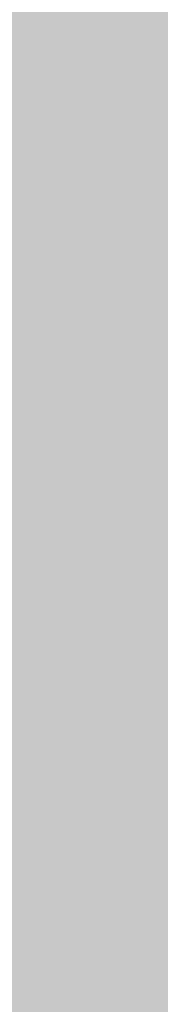
# Model space of a CAD drawing. Units: inches. Extents: x 2083 to 3317, y 1141 to 2115.
# Tile 188 of 256: x 3126.8914 to 3126.9283, y 1263.3548 to 1263.6134. Entities that reach past the tile are written whole.
import ezdxf

# ---------------------------------------------------------------- set-up
doc = ezdxf.new("R2010")
doc.units = ezdxf.units.IN
doc.layers.add('A-ANNO-DIMS', color=2, linetype='Continuous', lineweight=18)
doc.layers.add('A-WALL-PATT', color=251, linetype='Continuous', lineweight=13, true_color=0x636466)
doc.styles.get("Standard").update_dxf_attribs({"font": 'arial.ttf'})
doc.dimstyles.new('ISO-25', dxfattribs={"dimtxt": 12, "dimasz": 12, "dimexe": 1.25, "dimexo": 0.625, "dimtad": 1, "dimlunit": 3, "dimtxsty": 'Standard', "dimcen": 2.5, "dimadec": 0, "dimazin": 0, "dimtfac": 1, "dimtmove": 0, "dimatfit": 3, "dimfxl": 1, "dimarcsym": 0})

# ---------------------------------------------------------------- blocks, each defined once
blk = doc.blocks.new('*D26')
at = {"layer": 'A-ANNO-DIMS', "color": 0, "lineweight": -2, "transparency": 16777216}
for p, q in [((3088.98584, 1274.91509), (3088.98584, 1270.95196)), ((3111.24004, 1274.91509), (3111.24004, 1270.95196)), ((3076.98584, 1272.20196), (2840.26245, 1272.20196)), ((3111.24004, 1272.20196), (3088.98584, 1272.20196)), ((3123.24004, 1272.20196), (3135.24004, 1272.20196))]:
    blk.add_line(p, q, dxfattribs=at)
at = {"layer": 'A-ANNO-DIMS', "color": 0, "transparency": 16777216}
for points in [[(3076.98584, 1274.20196), (3076.98584, 1270.20196), (3088.98584, 1272.20196)], [(3123.24004, 1274.20196), (3123.24004, 1270.20196), (3111.24004, 1272.20196)]]:
    blk.add_solid(points, dxfattribs=at)
at = {"layer": 'Defpoints', "color": 0, "transparency": 16777216}
for p in [(3088.98584, 1275.54009), (3111.24004, 1275.54009), (3088.98584, 1272.20196)]:
    blk.add_point(p, dxfattribs=at)
at = {"layer": 'A-ANNO-DIMS', "color": 0, "transparency": 16777216, "insert": (2952.62415, 1279.0316), "char_height": 12, "attachment_point": 5}
blk.add_mtext('NIGHTSTAND 1\'-10 1/2" TYP.', dxfattribs=at)
blk = doc.blocks.new('*D27')
at = {"layer": 'A-ANNO-DIMS', "color": 0, "lineweight": -2, "transparency": 16777216}
for p, q in [((3114.57817, 1309.79428), (3114.57817, 1321.79428)), ((3111.86504, 1297.79428), (3115.82817, 1297.79428)), ((3114.57817, 1297.79428), (3114.57817, 1275.54009)), ((3111.86504, 1275.54009), (3115.82817, 1275.54009)), ((3114.57817, 1263.54009), (3114.57817, 1140.98859))]:
    blk.add_line(p, q, dxfattribs=at)
at = {"layer": 'A-ANNO-DIMS', "color": 0, "transparency": 16777216}
for points in [[(3112.57817, 1309.79428), (3116.57817, 1309.79428), (3114.57817, 1297.79428)], [(3112.57817, 1263.54009), (3116.57817, 1263.54009), (3114.57817, 1275.54009)]]:
    blk.add_solid(points, dxfattribs=at)
at = {"layer": 'Defpoints', "color": 0, "transparency": 16777216}
for p in [(3111.24004, 1297.79428), (3111.24004, 1275.54009), (3114.57817, 1275.54009)]:
    blk.add_point(p, dxfattribs=at)
at = {"layer": 'A-ANNO-DIMS', "color": 0, "transparency": 16777216, "insert": (3107.74853, 1196.26434), "char_height": 12, "attachment_point": 5, "rotation": 90}
blk.add_mtext('1\'-10 1/2" TYP.', dxfattribs=at)

msp = doc.modelspace()

# ---------------------------------------------------------------- hatches: boundary and pattern name
at = {"layer": 'A-WALL-PATT'}
h = msp.add_hatch(color=256, dxfattribs=at)
h.dxf.hatch_style = 1
h.paths.add_polyline_path([(3126.95978, 2020.76136), (2748.95978, 2020.76136), (2604.95978, 2020.76136), (2226.95978, 2020.76136), (2226.95978, 1702.76136), (2466.95978, 1702.76136), (2466.95978, 1582.76136), (2418.95978, 1582.76136), (2418.95978, 1477.76136), (2226.95978, 1477.76136), (2226.95978, 1263.26136), (2544.95978, 1263.26136), (2544.95978, 1411.76136), (2604.95978, 1411.76136), (2685.95978, 1411.76136), (2685.95978, 1420.76136), (2604.95978, 1420.76136), (2604.95978, 1573.76136), (2604.95978, 1702.76136), (2604.95978, 2011.76136), (2748.95978, 2011.76136), (2748.95978, 1702.76136), (2862.95978, 1702.76136), (2862.95978, 1621.76136), (2871.95978, 1621.76136), (2871.95978, 1702.76136), (2883.95978, 1702.76136), (2883.95978, 1706.93946, -0.026459), (2883.95978, 1711.76136), (2757.95978, 1711.76136), (2757.95978, 1807.76136), (2787.95978, 1807.76136), (2787.95978, 1812.26136), (2757.95978, 1812.26136), (2757.95978, 2011.76136), (2877.95978, 2011.76136), (2877.95978, 1812.26136), (2847.95978, 1812.26136), (2847.95978, 1807.76136), (2889.83574, 1807.76136), (2889.83574, 1812.26136), (2882.45978, 1812.26136), (2882.45978, 2011.76136), (3117.95978, 2011.76136), (3117.95978, 1812.26136), (2937.83574, 1812.26136), (2937.83574, 1807.76136), (2995.70978, 1807.76136), (2995.70978, 1796.11767), (3000.20978, 1796.11767), (3000.20978, 1807.76136), (3117.95978, 1807.76136), (3117.95978, 1711.76136), (3000.20978, 1711.76136), (3000.20978, 1760.11767), (2998.5727, 1760.11767, -0.020711), (2995.70978, 1760.11767), (2995.70978, 1711.76136), (2931.95978, 1711.76136), (2931.95978, 1702.76136), (3126.95978, 1702.76136)])
h.paths.add_polyline_path([(2471.45978, 2011.76136), (2471.45978, 1810.01136), (2462.71694, 1810.01136), (2462.71694, 1805.51136), (2505.95978, 1805.51136), (2505.95978, 1810.01136), (2475.95978, 1810.01136), (2475.95978, 2011.76136), (2595.95978, 2011.76136), (2595.95978, 1810.01136), (2565.95978, 1810.01136), (2565.95978, 1805.51136), (2595.95978, 1805.51136), (2595.95978, 1711.76136), (2235.95978, 1711.76136), (2235.95978, 1805.51136), (2353.70978, 1805.51136), (2353.70978, 1796.05416), (2358.20978, 1796.05416), (2358.20978, 1805.51136), (2414.71694, 1805.51136), (2414.71694, 1810.01136), (2235.95978, 1810.01136), (2235.95978, 2011.76136)], flags=16)
h.paths.add_polyline_path([(2270.20473, 1994.61001), (2270.20473, 1970.61001), (2246.20473, 1970.61001), (2246.20473, 1994.61001)], flags=0)
edge = h.paths.add_edge_path(flags=0)
edge.add_ellipse((2332.02739, 1899.79818), major_axis=(-3.04299, 3.04299), ratio=0.1682525, start_angle=-161.33217, end_angle=-156.30711, ccw=False)
edge.add_ellipse((2333.08204, 1898.74353), major_axis=(-1.05465, 1.05465), ratio=0.4535321, start_angle=-123.37102, end_angle=-94.15911)
edge = h.paths.add_edge_path(flags=0)
edge.add_ellipse((2332.02739, 1968.87629), major_axis=(3.04299, 3.04299), ratio=0.1682525, start_angle=18.66783, end_angle=23.69289)
edge.add_spline(control_points=[(2332.9256, 1970.6911), (2332.22677, 1970.3361), (2330.89371, 1969.65891), (2328.41308, 1970.93214), (2327.20393, 1967.74871), (2324.7096, 1969.95559), (2322.53282, 1967.01235), (2320.01285, 1971.29581), (2317.68031, 1968.15784), (2316.04053, 1967.10205), (2315.4269, 1966.8096)], knot_values=[0, 0, 0, 0, 2.267059, 4.324559, 6.685584, 8.878641, 11.121502, 14.300359, 17.755284, 19.732645, 19.732645, 19.732645, 19.732645], degree=3, periodic=0)
edge.add_ellipse((2332.02739, 1968.87629), major_axis=(3.04299, 3.04299), ratio=0.1682525, start_angle=18.66783, end_angle=23.69289, ccw=False)
edge.add_ellipse((2333.08204, 1969.93094), major_axis=(1.05465, 1.05465), ratio=0.4535321, start_angle=56.62898, end_angle=85.84089, ccw=False)
edge = h.paths.add_edge_path(flags=0)
edge.add_spline(control_points=[(2296.42829, 1967.98791), (2293.6278, 1965.33631), (2287.70362, 1959.72709), (2299.74386, 1949.9957), (2294.53259, 1935.66853), (2290.57323, 1920.60351), (2293.39412, 1909.97369), (2296.18541, 1904.96654)], knot_values=[0.099185, 0.099185, 0.099185, 0.099185, 0.345301, 0.619822, 0.982653, 1.386093, 1.810555, 1.810555, 1.810555, 1.810555], degree=3, periodic=0)
edge.add_spline(control_points=[(2296.18541, 1904.96654), (2297.38358, 1902.6193), (2298.00097, 1901.94931), (2298.55297, 1901.46815)], knot_values=[0.006246, 0.006246, 0.006246, 0.006246, 0.055476, 0.055476, 0.055476, 0.055476], degree=3, periodic=0)
edge.add_spline(control_points=[(2298.55297, 1901.46815), (2297.25861, 1900.92322), (2295.22529, 1900.23213), (2293.06023, 1900.61421), (2292.10142, 1900.78841), (2292.08958, 1900.79057)], knot_values=[0.312835, 0.312835, 0.312835, 0.312835, 0.40178, 0.474987, 0.475903, 0.475903, 0.475903, 0.475903], degree=3, periodic=0)
edge.add_arc((2292.79365, 1904.66411), 3.93701, 215.4209, 259.69818, ccw=False)
edge.add_spline(control_points=[(2289.58531, 1902.3823), (2289.47665, 1902.53509), (2289.36848, 1902.68804), (2289.26086, 1902.84117)], knot_values=[0.102872, 0.102872, 0.102872, 0.102872, 0.116896, 0.116896, 0.116896, 0.116896], degree=3, periodic=0)
edge.add_spline(control_points=[(2289.26086, 1902.84117), (2288.6866, 1902.55019), (2287.64005, 1902.0199), (2285.88134, 1901.87395), (2283.85297, 1901.50435), (2281.71999, 1899.71054), (2278.46699, 1899.49294), (2276.15714, 1901.8832), (2272.25895, 1899.80407), (2267.77761, 1901.84318), (2262.24388, 1900.18403), (2257.41493, 1901.78206), (2254.31837, 1900.72612), (2253.17828, 1900.33734)], knot_values=[0, 0, 0, 0, 1.907977, 3.477176, 5.261074, 7.972851, 11.680248, 13.717921, 16.939592, 22.789562, 27.502503, 33.595215, 37.145618, 37.145618, 37.145618, 37.145618], degree=3, periodic=0)
edge.add_line((2253.17828, 1900.33734), (2250.24424, 1902.84117))
edge.add_line((2250.24424, 1902.84117), (2250.24424, 1965.8333))
edge.add_line((2250.24424, 1965.8333), (2253.17828, 1968.33712))
edge.add_spline(control_points=[(2253.17828, 1968.33712), (2254.31837, 1967.94835), (2257.41493, 1966.89241), (2262.24388, 1968.49043), (2267.77761, 1966.83128), (2271.52673, 1968.53722), (2273.87591, 1967.82829), (2274.2067, 1967.72764)], knot_values=[0, 0, 0, 0, 0.09018, 0.244935, 0.364644, 0.513233, 0.537855, 0.537855, 0.537855, 0.537855], degree=3, periodic=0)
edge.add_arc((2274.35289, 1963.79335), 3.93701, 72.05113, 92.12795, ccw=False)
edge.add_arc((2281.29693, 1985.23), 18.5963, 252.051134, 288.565722)
edge.add_arc((2292.31672, 1956.02888), 12.64608, 71.026788, 113.778218, ccw=False)
edge = h.paths.add_edge_path(flags=0)
edge.add_spline(control_points=[(2274.89941, 1951.85619), (2275.06616, 1951.61659), (2275.23269, 1951.37659), (2275.39799, 1951.13585)], knot_values=[1.409916, 1.409916, 1.409916, 1.409916, 1.43159, 1.43159, 1.43159, 1.43159], degree=3, periodic=0)
edge.add_spline(control_points=[(2275.39799, 1951.13585), (2275.79211, 1950.56189), (2276.17923, 1949.98377), (2276.54555, 1949.3971)], knot_values=[1.358238, 1.358238, 1.358238, 1.358238, 1.409916, 1.409916, 1.409916, 1.409916], degree=3, periodic=0)
edge.add_line((2276.54555, 1949.3971), (2277.43729, 1947.86218))
edge.add_spline(control_points=[(2277.43729, 1947.86218), (2276.30383, 1945.67311), (2274.6397, 1942.42688), (2274.63161, 1938.0939), (2272.79912, 1930.85155), (2274.35643, 1943.89705), (2275.94768, 1947.92336), (2276.54555, 1949.3971)], knot_values=[0.005632, 0.005632, 0.005632, 0.005632, 0.186014, 0.266002, 0.357087, 0.59639, 0.739732, 0.739732, 0.739732, 0.739732], degree=3, periodic=0)
edge.add_spline(control_points=[(2276.54555, 1949.3971), (2276.17923, 1949.98377), (2275.79211, 1950.56189), (2275.39799, 1951.13585)], knot_values=[1.358238, 1.358238, 1.358238, 1.358238, 1.409916, 1.409916, 1.409916, 1.409916], degree=3, periodic=0)
edge.add_spline(control_points=[(2275.39799, 1951.13585), (2274.9425, 1950.08045), (2274.20776, 1948.02527), (2273.9346, 1944.85148), (2272.46853, 1937.62749), (2273.46622, 1945.69647), (2274.70062, 1951.05947), (2274.89941, 1951.85619)], knot_values=[0.104364, 0.104364, 0.104364, 0.104364, 0.189636, 0.269624, 0.36071, 0.600013, 0.644622, 0.644622, 0.644622, 0.644622], degree=3, periodic=0)
h.paths.add_polyline_path([(2269.16751, 1963.12757, -0.357527), (2268.17063, 1960.97637, -0.092561), (2268.17063, 1939.43632, -0.357527), (2269.16751, 1937.28512, -0.357527), (2267.01631, 1938.282, -0.164785), (2254.68558, 1938.282, -0.357527), (2252.53438, 1937.28512, -0.357527), (2253.53126, 1939.43632, -0.092561), (2253.53126, 1960.97637, -0.357527), (2252.53438, 1963.12757, -0.357527), (2254.68558, 1962.13069, -0.164785), (2267.01631, 1962.13069, -0.357527)], flags=0)
h.paths.add_polyline_path([(2248.87407, 1967.8018), (2248.87407, 1957.02771), (2249.45778, 1957.02771), (2249.45778, 1911.64676), (2248.87407, 1911.64676), (2248.87407, 1900.87267), (2246.51186, 1900.87267, 0.197327), (2244.14966, 1902.45687), (2244.14966, 1966.21759, 0.197327), (2246.51186, 1967.8018)], flags=0)
h.paths.add_polyline_path([(2269.16751, 1931.38934, -0.357527), (2268.17063, 1929.23814, -0.092561), (2268.17063, 1907.6981, -0.357527), (2269.16751, 1905.54689, -0.357527), (2267.01631, 1906.54377, -0.164785), (2254.68558, 1906.54377, -0.357527), (2252.53438, 1905.54689, -0.357527), (2253.53126, 1907.6981, -0.092561), (2253.53126, 1929.23814, -0.357527), (2252.53438, 1931.38934, -0.357527), (2254.68558, 1930.39246, -0.164785), (2267.01631, 1930.39246, -0.357527)], flags=0)
edge = h.paths.add_edge_path(flags=0)
edge.add_spline(control_points=[(2276.19686, 1906.7237), (2276.16814, 1909.02893), (2276.11405, 1913.37185), (2270.59842, 1924.92498), (2273.90517, 1919.01278), (2275.92171, 1916.26206), (2275.47457, 1912.40215), (2277.25787, 1910.38062), (2276.69604, 1908.22504), (2276.64622, 1906.81302), (2276.61782, 1906.00841)], knot_values=[0, 0, 0, 0, 8.61026, 16.221274, 18.843057, 23.804898, 27.440828, 29.356102, 31.203478, 33.650687, 33.650687, 33.650687, 33.650687], degree=3, periodic=0)
edge.add_spline(control_points=[(2276.61782, 1906.00841), (2276.62331, 1905.62414), (2276.49774, 1904.62866), (2275.44178, 1903.85473), (2274.93731, 1903.08045), (2274.85908, 1902.84117)], knot_values=[0.156488, 0.156488, 0.156488, 0.156488, 0.184398, 0.231376, 0.250598, 0.250598, 0.250598, 0.250598], degree=3, periodic=0)
edge.add_line((2274.85908, 1902.84117), (2276.50598, 1902.84117))
edge.add_spline(control_points=[(2276.50598, 1902.84117), (2276.78831, 1903.08494), (2277.66507, 1904.1252), (2278.24954, 1904.34074), (2277.65387, 1908.52739), (2278.15567, 1906.22781), (2278.10046, 1905.28595), (2278.84667, 1904.06901), (2277.85679, 1903.41495), (2277.87419, 1902.99105), (2277.90356, 1902.84117)], knot_values=[0.059574, 0.059574, 0.059574, 0.059574, 0.080753, 0.103741, 0.16972, 0.176036, 0.207137, 0.240474, 0.262341, 0.27366, 0.27366, 0.27366, 0.27366], degree=3, periodic=0)
edge.add_line((2277.90356, 1902.84117), (2280.02983, 1902.84117))
edge.add_spline(control_points=[(2280.02983, 1902.84117), (2279.88822, 1903.0884), (2279.49926, 1903.98155), (2280.15228, 1905.93935), (2278.10362, 1909.65776), (2279.76239, 1907.18529), (2280.3279, 1904.87486), (2280.48511, 1903.48959), (2281.46327, 1903.24943), (2281.75834, 1902.9365), (2281.83404, 1902.84117)], knot_values=[0.013856, 0.013856, 0.013856, 0.013856, 0.034874, 0.088867, 0.107879, 0.126738, 0.158714, 0.193757, 0.217487, 0.226722, 0.226722, 0.226722, 0.226722], degree=3, periodic=0)
edge.add_spline(control_points=[(2281.83404, 1902.84117), (2281.78753, 1902.8267), (2281.64702, 1902.78299), (2281.39553, 1902.85949), (2281.08808, 1902.98524), (2280.72068, 1903.0609), (2280.33345, 1903.02573), (2280.12477, 1902.89888), (2280.02983, 1902.84117)], knot_values=[0, 0, 0, 0, 0.14413, 0.435517, 0.749276, 1.153046, 1.548371, 1.878348, 1.878348, 1.878348, 1.878348], degree=3, periodic=0)
edge.add_line((2280.02983, 1902.84117), (2277.90356, 1902.84117))
edge.add_spline(control_points=[(2277.90356, 1902.84117), (2277.89286, 1902.79586), (2277.8654, 1902.67964), (2277.60748, 1902.68748), (2277.27405, 1902.8007), (2276.83792, 1902.61977), (2276.58381, 1902.78926), (2276.50598, 1902.84117)], knot_values=[0, 0, 0, 0, 0.127189, 0.326199, 0.628009, 1.24357, 1.515331, 1.515331, 1.515331, 1.515331], degree=3, periodic=0)
edge.add_line((2276.50598, 1902.84117), (2274.85908, 1902.84117))
edge.add_spline(control_points=[(2274.85908, 1902.84117), (2274.81444, 1902.89859), (2274.72513, 1903.01345), (2274.49348, 1903.11897), (2274.24429, 1902.96054), (2273.93712, 1903.18494), (2273.61404, 1902.98314), (2273.40832, 1902.88304), (2273.32225, 1902.84117)], knot_values=[0, 0, 0, 0, 0.21843, 0.436957, 0.687977, 0.990379, 1.398396, 1.69185, 1.69185, 1.69185, 1.69185], degree=3, periodic=0)
edge.add_spline(control_points=[(2273.32225, 1902.84117), (2273.61674, 1903.44569), (2274.274, 1904.53825), (2276.02724, 1904.5737), (2276.20696, 1906.58364), (2276.19686, 1906.7237)], knot_values=[0.012227, 0.012227, 0.012227, 0.012227, 0.059472, 0.106218, 0.134458, 0.134458, 0.134458, 0.134458], degree=3, periodic=0)
h.paths.add_polyline_path([(2270.77605, 1897.78983), (2270.77605, 1873.78983), (2246.77605, 1873.78983), (2246.77605, 1897.78983)], flags=0)
h.paths.add_polyline_path([(2353.70978, 1760.00506), (2353.70978, 1760.05416), (2358.20978, 1760.05416, -0.033729)], flags=0)
h.paths.add_polyline_path([(2321.81912, 1737.52919), (2341.99533, 1737.52919, -0.414214), (2343.20327, 1736.32124), (2343.20327, 1721.0206, -0.414214), (2341.99533, 1719.81265), (2321.81912, 1719.81265, -0.414214), (2320.61117, 1721.0206), (2320.61117, 1736.32124, -0.414214)], flags=0)
h.paths.add_polyline_path([(2324.23501, 1736.32124), (2339.57944, 1736.32124, -0.414214), (2341.99533, 1733.90535), (2341.99533, 1725.44973, -0.414214), (2339.57944, 1723.03384), (2333.68059, 1723.03384), (2333.84532, 1722.04547, -0.870646), (2335.4254, 1721.82589, -0.767327), (2333.92269, 1721.42324), (2331.29102, 1721.42324, -0.767327), (2329.78832, 1721.82589, -0.870646), (2331.3684, 1722.04547), (2331.53313, 1723.03384), (2324.23501, 1723.03384, -0.414214), (2321.81912, 1725.44973), (2321.81912, 1733.90535, -0.414214)], flags=0)
h.paths.add_polyline_path([(2570.48379, 1928.61544), (2589.68379, 1928.61544), (2590.16883, 1928.61544), (2590.16883, 1904.9934), (2570.48379, 1904.9934)], flags=0)
h.paths.add_polyline_path([(2574.44732, 1927.26382, -1), (2572.82884, 1927.26382, -1)], flags=0)
h.paths.add_polyline_path([(2573.08987, 1926.94088), (2573.92503, 1927.77604), (2574.14774, 1927.55333), (2573.31258, 1926.71817)], flags=0)
h.paths.add_polyline_path([(2578.77906, 1919.72962, -1), (2571.59166, 1919.72962, -1)], flags=0)
h.paths.add_polyline_path([(2578.38536, 1919.72962, -1), (2571.98536, 1919.72962, -1)], flags=0)
h.paths.add_polyline_path([(2331.59576, 1729.47622, -1), (2333.61795, 1729.47622, -1)], flags=0)
h.paths.add_polyline_path([(2578.03423, 1927.26382, -1), (2576.41574, 1927.26382, -1)], flags=0)
h.paths.add_polyline_path([(2576.68885, 1927.53109), (2576.91156, 1927.7538), (2577.74673, 1926.91863), (2577.52402, 1926.69592)], flags=0)
h.paths.add_polyline_path([(2578.13906, 1909.85954, -1), (2572.23166, 1909.85954, -1)], flags=0)
h.paths.add_polyline_path([(2577.74536, 1909.85954, -1), (2572.62536, 1909.85954, -1)], flags=0)
h.paths.add_polyline_path([(2583.79772, 1927.26382, -1), (2582.17923, 1927.26382, -1)], flags=0)
h.paths.add_polyline_path([(2582.71865, 1927.7538), (2583.55381, 1926.91863), (2583.3311, 1926.69592), (2582.49594, 1927.53109)], flags=0)
h.paths.add_polyline_path([(2582.49594, 1927.53109), (2582.71865, 1927.7538), (2583.55381, 1926.91863), (2583.3311, 1926.69592)], flags=0)
h.paths.add_polyline_path([(2587.73906, 1920.52962, -1), (2581.83166, 1920.52962, -1)], flags=0)
h.paths.add_polyline_path([(2587.34536, 1920.52962, -1), (2582.22536, 1920.52962, -1)], flags=0)
h.paths.add_polyline_path([(2587.38462, 1927.26382, -1), (2585.76613, 1927.26382, -1)], flags=0)
h.paths.add_polyline_path([(2586.08199, 1926.98025), (2586.91716, 1927.81541), (2587.13987, 1927.5927), (2586.3047, 1926.75754)], flags=0)
h.paths.add_polyline_path([(2588.37906, 1910.65954, -1), (2581.19166, 1910.65954, -1)], flags=0)
h.paths.add_polyline_path([(2587.98536, 1910.65954, -1), (2581.58536, 1910.65954, -1)], flags=0)
h.paths.add_polyline_path([(2417.16773, 1729.4779), (2437.34394, 1729.4779, -0.414214), (2438.55188, 1728.26995), (2438.55188, 1712.96931, -0.414214), (2437.34394, 1711.76136), (2417.16773, 1711.76136, -0.414214), (2415.95978, 1712.96931), (2415.95978, 1728.26995, -0.414214)], flags=0)
h.paths.add_polyline_path([(2419.58362, 1728.26995), (2434.92805, 1728.26995, -0.414214), (2437.34394, 1725.85406), (2437.34394, 1717.39844, -0.414214), (2434.92805, 1714.98255), (2429.0292, 1714.98255), (2429.19393, 1713.99418, -0.870646), (2430.77401, 1713.7746, -0.767327), (2429.2713, 1713.37195), (2426.63963, 1713.37195, -0.767327), (2425.13693, 1713.7746, -0.870646), (2426.71701, 1713.99418), (2426.88174, 1714.98255), (2419.58362, 1714.98255, -0.414214), (2417.16773, 1717.39844), (2417.16773, 1725.85406, -0.414214)], flags=0)
h.paths.add_polyline_path([(2419.58362, 1728.26995), (2434.92805, 1728.26995, -0.414214), (2437.34394, 1725.85406), (2437.34394, 1717.39844, -0.414214), (2434.92805, 1714.98255), (2429.0292, 1714.98255), (2428.35812, 1719.00903), (2427.55282, 1719.00903), (2426.88174, 1714.98255), (2419.58362, 1714.98255, -0.414214), (2417.16773, 1717.39844), (2417.16773, 1725.85406, -0.414214)], flags=0)
h.paths.add_polyline_path([(2426.94437, 1721.42492, -1), (2428.96656, 1721.42492, -1)], flags=0)
h.paths.add_polyline_path([(2475.95978, 1702.76136), (2595.95978, 1702.76136), (2595.95978, 1582.76136), (2475.95978, 1582.76136)], flags=16)
h.paths.add_polyline_path([(2427.95978, 1573.76136), (2595.95978, 1573.76136), (2595.95978, 1468.76136), (2595.95978, 1420.76136), (2384.45978, 1420.76136), (2384.45978, 1468.76136), (2427.95978, 1468.76136)], flags=16)
h.paths.add_polyline_path([(2379.95978, 1468.76136), (2379.95978, 1420.76136), (2235.95978, 1420.76136), (2235.95978, 1468.76136)], flags=16)
h.paths.add_polyline_path([(2317.816, 1466.69577), (2337.9922, 1466.69577, -0.414214), (2339.20015, 1465.48782), (2339.20015, 1450.18718, -0.414214), (2337.9922, 1448.97923), (2317.816, 1448.97923, -0.414214), (2316.60805, 1450.18718), (2316.60805, 1465.48782, -0.414214)], flags=0)
h.paths.add_polyline_path([(2320.23189, 1465.48782), (2335.57631, 1465.48782, -0.414214), (2337.9922, 1463.07193), (2337.9922, 1454.61631, -0.414214), (2335.57631, 1452.20042), (2329.67747, 1452.20042), (2329.84219, 1451.21205, -0.870646), (2331.42228, 1450.99247, -0.767327), (2329.91957, 1450.58983), (2327.2879, 1450.58983, -0.767327), (2325.7852, 1450.99247, -0.870646), (2327.36528, 1451.21205), (2327.53001, 1452.20042), (2320.23189, 1452.20042, -0.414214), (2317.816, 1454.61631), (2317.816, 1463.07193, -0.414214)], flags=0)
h.paths.add_polyline_path([(2320.23189, 1465.48782), (2335.57631, 1465.48782, -0.414214), (2337.9922, 1463.07193), (2337.9922, 1454.61631, -0.414214), (2335.57631, 1452.20042), (2329.67747, 1452.20042), (2329.00638, 1456.22691), (2328.20109, 1456.22691), (2327.53001, 1452.20042), (2320.23189, 1452.20042, -0.414214), (2317.816, 1454.61631), (2317.816, 1463.07193, -0.414214)], flags=0)
h.paths.add_polyline_path([(2327.59264, 1458.6428, -1), (2329.61483, 1458.6428, -1)], flags=0)
h.paths.add_polyline_path([(2244.41174, 1433.34045), (2241.92094, 1433.34045, -0.414214), (2240.01786, 1435.24354), (2240.01786, 1440.95281, -0.414211), (2241.92093, 1442.8559), (2244.41174, 1442.8559, -1.976472)], flags=0)
h.paths.add_polyline_path([(2245.35689, 1434.39754, -0.414214), (2245.35689, 1441.79881, -2.144098)], flags=0)
h.paths.add_polyline_path([(2535.95978, 1416.26136), (2535.95978, 1272.26136), (2235.95978, 1272.26136), (2235.95978, 1416.26136)], flags=16)
h.paths.add_polyline_path([(2260.11956, 1384.29284), (2260.11956, 1362.03865), (2237.86537, 1362.03865), (2237.86537, 1384.29284)], flags=0)
edge = h.paths.add_edge_path(flags=0)
edge.add_line((2318.25185, 1362.0933), (2318.1458, 1362.00097))
edge.add_ellipse((2317.44512, 1360.43104), major_axis=(2.82164, 2.82164), ratio=0.1682525, start_angle=18.66783, end_angle=20.94813, ccw=False)
edge.add_ellipse((2318.42305, 1361.40897), major_axis=(0.97793, 0.97793), ratio=0.4535321, start_angle=56.62898, end_angle=70.2262, ccw=False)
edge = h.paths.add_edge_path(flags=0)
edge.add_line((2319.10737, 1295.57108), (2319.01504, 1295.67713))
edge.add_ellipse((2317.44512, 1296.37781), major_axis=(-2.82164, 2.82164), ratio=0.1682525, start_angle=-161.33217, end_angle=-159.05187, ccw=False)
edge.add_ellipse((2318.42305, 1295.39988), major_axis=(-0.97793, 0.97793), ratio=0.4535321, start_angle=-123.37102, end_angle=-109.7738)
edge = h.paths.add_edge_path(flags=0)
edge.add_spline(control_points=[(2284.21035, 1301.17022), (2284.58069, 1300.44472), (2284.89119, 1299.89202), (2285.15955, 1299.46102)], knot_values=[0.039066, 0.039066, 0.039066, 0.039066, 0.055476, 0.055476, 0.055476, 0.055476], degree=3, periodic=0)
edge.add_line((2285.15955, 1299.46102), (2284.21035, 1301.17022))
edge = h.paths.add_edge_path(flags=0)
edge.add_line((2280.41246, 1297.29801), (2283.36999, 1297.03612))
edge.add_line((2283.36999, 1297.03612), (2286.40569, 1297.92631))
edge.add_spline(control_points=[(2286.40569, 1297.92631), (2285.30549, 1297.46312), (2284.34478, 1297.12915), (2283.36999, 1297.03612)], knot_values=[0.394369, 0.394369, 0.394369, 0.394369, 0.475903, 0.475903, 0.475903, 0.475903], degree=3, periodic=0)
edge.add_spline(control_points=[(2283.36999, 1297.03612), (2283.28139, 1297.02767), (2282.31629, 1296.95734), (2281.3125, 1297.13448), (2280.42344, 1297.29602), (2280.41246, 1297.29801)], knot_values=[0.312835, 0.312835, 0.312835, 0.312835, 0.320246, 0.393453, 0.394369, 0.394369, 0.394369, 0.394369], degree=3, periodic=0)
edge = h.paths.add_edge_path(flags=0)
edge.add_line((2284.43556, 1359.60729), (2280.44629, 1355.32805))
edge.add_line((2280.44629, 1355.32805), (2279.57999, 1351.01775))
edge.add_line((2279.57999, 1351.01775), (2282.41297, 1346.58043))
edge.add_spline(control_points=[(2282.41297, 1346.58043), (2283.15333, 1345.58924), (2284.2529, 1344.0289), (2284.80104, 1342.38717), (2284.93516, 1341.80554)], knot_values=[1.240098, 1.240098, 1.240098, 1.240098, 1.332892, 1.382712, 1.382712, 1.382712, 1.382712], degree=3, periodic=0)
edge.add_spline(control_points=[(2284.93516, 1341.80554), (2285.31911, 1340.1406), (2285.23303, 1338.4092), (2284.90994, 1336.65412)], knot_values=[1.097484, 1.097484, 1.097484, 1.097484, 1.240098, 1.240098, 1.240098, 1.240098], degree=3, periodic=0)
edge.add_spline(control_points=[(2284.90994, 1336.65412), (2284.58685, 1334.89904), (2284.02675, 1333.12027), (2283.46264, 1331.36058)], knot_values=[0.95487, 0.95487, 0.95487, 0.95487, 1.097484, 1.097484, 1.097484, 1.097484], degree=3, periodic=0)
edge.add_line((2283.46264, 1331.36058), (2281.89038, 1326.15336))
edge.add_line((2281.89038, 1326.15336), (2280.75626, 1321.05609))
edge.add_line((2280.75626, 1321.05609), (2280.2992, 1316.00198))
edge.add_line((2280.2992, 1316.00198), (2280.71593, 1310.95007))
edge.add_line((2280.71593, 1310.95007), (2282.02809, 1305.97214))
edge.add_line((2282.02809, 1305.97214), (2284.21035, 1301.17022))
edge.add_spline(control_points=[(2284.21035, 1301.17022), (2283.34073, 1302.73019), (2282.6119, 1304.33649), (2282.02809, 1305.97214)], knot_values=[0.099185, 0.099185, 0.099185, 0.099185, 0.241799, 0.241799, 0.241799, 0.241799], degree=3, periodic=0)
edge.add_spline(control_points=[(2282.02809, 1305.97214), (2281.44428, 1307.60778), (2281.00549, 1309.27276), (2280.71593, 1310.95007)], knot_values=[0.241799, 0.241799, 0.241799, 0.241799, 0.384413, 0.384413, 0.384413, 0.384413], degree=3, periodic=0)
edge.add_spline(control_points=[(2280.71593, 1310.95007), (2280.43324, 1312.58761), (2280.28939, 1314.27696), (2280.29889, 1315.96203), (2280.2992, 1316.00198)], knot_values=[0.384413, 0.384413, 0.384413, 0.384413, 0.523647, 0.527028, 0.527028, 0.527028, 0.527028], degree=3, periodic=0)
edge.add_spline(control_points=[(2280.2992, 1316.00198), (2280.31233, 1317.68696), (2280.47787, 1319.36793), (2280.75626, 1321.05609)], knot_values=[0.527028, 0.527028, 0.527028, 0.527028, 0.669642, 0.669642, 0.669642, 0.669642], degree=3, periodic=0)
edge.add_spline(control_points=[(2280.75626, 1321.05609), (2281.03465, 1322.74425), (2281.42588, 1324.43961), (2281.89038, 1326.15336)], knot_values=[0.669642, 0.669642, 0.669642, 0.669642, 0.812256, 0.812256, 0.812256, 0.812256], degree=3, periodic=0)
edge.add_spline(control_points=[(2281.89038, 1326.15336), (2282.26438, 1327.53325), (2282.78787, 1329.26181), (2283.35275, 1331.01778), (2283.46264, 1331.36058)], knot_values=[0.812256, 0.812256, 0.812256, 0.812256, 0.927087, 0.95487, 0.95487, 0.95487, 0.95487], degree=3, periodic=0)
edge.add_line((2283.46264, 1331.36058), (2284.90994, 1336.65412))
edge.add_line((2284.90994, 1336.65412), (2284.93516, 1341.80554))
edge.add_line((2284.93516, 1341.80554), (2282.41297, 1346.58043))
edge.add_spline(control_points=[(2282.41297, 1346.58043), (2281.27513, 1348.10379), (2280.07845, 1349.57032), (2279.57999, 1351.01775)], knot_values=[1.382712, 1.382712, 1.382712, 1.382712, 1.525326, 1.525326, 1.525326, 1.525326], degree=3, periodic=0)
edge.add_spline(control_points=[(2279.57999, 1351.01775), (2279.44328, 1351.41472), (2279.13631, 1352.85692), (2279.73519, 1354.29039), (2280.44629, 1355.32805)], knot_values=[1.525326, 1.525326, 1.525326, 1.525326, 1.564439, 1.667941, 1.667941, 1.667941, 1.667941], degree=3, periodic=0)
edge.add_spline(control_points=[(2280.44629, 1355.32805), (2281.42611, 1356.75784), (2282.93084, 1358.18256), (2284.43556, 1359.60729)], knot_values=[1.667941, 1.667941, 1.667941, 1.667941, 1.810555, 1.810555, 1.810555, 1.810555], degree=3, periodic=0)
edge.add_arc((2280.62307, 1348.51818), 11.72618, 71.026788, 113.778218)
edge.add_arc((2270.40489, 1375.59516), 17.24357, 252.051134, 288.565722, ccw=False)
edge.add_arc((2263.96597, 1355.71785), 3.65062, 72.05113, 92.12795)
edge.add_arc((2263.96597, 1355.71785), 3.65062, 92.12795, 177.98513)
edge.add_spline(control_points=[(2260.3176, 1355.8462), (2260.26042, 1354.22067), (2260.55128, 1350.18655), (2262.99934, 1346.76625), (2264.47274, 1344.64902)], knot_values=[1.43159, 1.43159, 1.43159, 1.43159, 1.564144, 1.770695, 1.770695, 1.770695, 1.770695], degree=3, periodic=0)
edge.add_line((2264.47274, 1344.64902), (2264.93559, 1343.98253))
edge.add_spline(control_points=[(2263.80104, 1340.24811), (2263.84324, 1340.51409), (2264.06724, 1341.75647), (2264.51269, 1343.00245), (2264.93505, 1343.98108)], knot_values=[0.53657, 0.53657, 0.53657, 0.53657, 0.559349, 0.644622, 0.644622, 0.644622, 0.644622], degree=3, periodic=0)
edge.add_spline(control_points=[(2264.93505, 1343.98108), (2265.11777, 1343.71497), (2265.29888, 1343.44791), (2265.47676, 1343.17936)], knot_values=[1.384077, 1.384077, 1.384077, 1.384077, 1.409916, 1.409916, 1.409916, 1.409916], degree=3, periodic=0)
edge.add_spline(control_points=[(2265.47676, 1343.17936), (2265.65464, 1342.91082), (2265.8293, 1342.64081), (2265.99913, 1342.36881)], knot_values=[1.358238, 1.358238, 1.358238, 1.358238, 1.384077, 1.384077, 1.384077, 1.384077], degree=3, periodic=0)
edge.add_line((2265.99913, 1342.36881), (2266.82601, 1340.94555))
edge.add_spline(control_points=[(2266.82601, 1340.94555), (2268.8944, 1337.08969), (2271.39817, 1325.843), (2270.51616, 1310.56856), (2275.91938, 1301.86061), (2277.78951, 1299.19945)], knot_values=[0.116896, 0.116896, 0.116896, 0.116896, 0.472987, 1.050969, 1.313793, 1.313793, 1.313793, 1.313793], degree=3, periodic=0)
edge.add_spline(control_points=[(2277.78951, 1299.19945), (2277.83941, 1299.12845), (2277.88943, 1299.0575), (2277.93957, 1298.98658)], knot_values=[0.109884, 0.109884, 0.109884, 0.109884, 0.116896, 0.116896, 0.116896, 0.116896], degree=3, periodic=0)
edge.add_line((2277.93957, 1298.98658), (2277.78885, 1299.19911))
edge.add_spline(control_points=[(2277.78885, 1299.19911), (2277.25658, 1298.92941), (2276.28635, 1298.4379), (2275.03935, 1298.33442), (2274.38333, 1298.2389), (2274.21525, 1298.20934)], knot_values=[33.12187, 33.12187, 33.12187, 33.12187, 35.029056, 36.598255, 37.144827, 37.144827, 37.144827, 37.144827], degree=3, periodic=0)
edge.add_line((2274.21525, 1298.20934), (2273.07315, 1297.89296))
edge.add_spline(control_points=[(2273.07315, 1297.89296), (2272.32294, 1297.57978), (2271.03915, 1296.51051), (2269.24839, 1296.22606), (2268.4231, 1296.37465)], knot_values=[26.532584, 26.532584, 26.532584, 26.532584, 29.198919, 31.839101, 31.839101, 31.839101, 31.839101], degree=3, periodic=0)
edge.add_line((2268.4231, 1296.37465), (2263.8785, 1297.45753))
edge.add_spline(control_points=[(2263.8785, 1297.45753), (2263.55608, 1297.35943), (2261.86031, 1296.83869), (2260.23878, 1297.28241), (2258.93345, 1297.51646)], knot_values=[15.919551, 15.919551, 15.919551, 15.919551, 16.939592, 21.226067, 21.226067, 21.226067, 21.226067], degree=3, periodic=0)
edge.add_line((2258.93345, 1297.51646), (2254.05523, 1297.32901))
edge.add_spline(control_points=[(2254.05523, 1297.32901), (2253.75553, 1297.29582), (2252.11368, 1297.16517), (2250.46187, 1297.54422), (2249.12969, 1297.66788)], knot_values=[5.306517, 5.306517, 5.306517, 5.306517, 6.276435, 10.613034, 10.613034, 10.613034, 10.613034], degree=3, periodic=0)
edge.add_line((2249.12969, 1297.66788), (2244.33165, 1296.87776))
edge.add_line((2244.33165, 1296.87776), (2241.61103, 1299.19945))
edge.add_line((2241.61103, 1299.19945), (2241.61103, 1357.6094))
edge.add_line((2241.61103, 1357.6094), (2244.33165, 1359.9311))
edge.add_line((2244.33165, 1359.9311), (2252.72882, 1359.54269))
edge.add_spline(control_points=[(2252.72882, 1359.54269), (2252.87094, 1359.54644), (2253.30574, 1359.54817), (2253.73984, 1359.51427), (2254.03174, 1359.48243)], knot_values=[0.233291, 0.233291, 0.233291, 0.233291, 0.244935, 0.268927, 0.268927, 0.268927, 0.268927], degree=3, periodic=0)
edge.add_line((2254.03174, 1359.48243), (2259.58719, 1359.41639))
edge.add_spline(control_points=[(2259.58719, 1359.41639), (2260.67707, 1359.6285), (2262.0732, 1359.897), (2263.52369, 1359.45928), (2263.83042, 1359.36595)], knot_values=[0.422516, 0.422516, 0.422516, 0.422516, 0.513233, 0.537855, 0.537855, 0.537855, 0.537855], degree=3, periodic=0)
edge.add_arc((2263.96597, 1355.71785), 3.65062, 72.05113, 92.12795, ccw=False)
edge.add_arc((2270.40489, 1375.59516), 17.24357, 252.051134, 288.565722)
edge.add_arc((2280.62307, 1348.51818), 11.72618, 71.026788, 113.778218, ccw=False)
h.paths.add_polyline_path([(2240.34053, 1359.43471), (2240.34053, 1349.44435), (2240.88178, 1349.44435), (2240.88178, 1307.3645), (2240.34053, 1307.3645), (2240.34053, 1297.37414), (2238.15016, 1297.37414, 0.197327), (2235.95978, 1298.84311), (2235.95978, 1357.96575, 0.197327), (2238.15016, 1359.43471)], flags=0)
h.paths.add_polyline_path([(2259.15779, 1355.1005, -0.357527), (2258.23342, 1353.10578, -0.092561), (2258.23342, 1333.1326, -0.357527), (2259.15779, 1331.13788, -0.357527), (2257.16307, 1332.06225, -0.164785), (2245.7293, 1332.06225, -0.357527), (2243.73458, 1331.13788, -0.357527), (2244.65895, 1333.1326, -0.092561), (2244.65895, 1353.10578, -0.357527), (2243.73458, 1355.1005, -0.357527), (2245.7293, 1354.17613, -0.164785), (2257.16307, 1354.17613, -0.357527)], flags=0)
edge = h.paths.add_edge_path(flags=0)
edge.add_line((2265.99913, 1342.36881), (2266.82601, 1340.94555))
edge.add_line((2266.82601, 1340.94555), (2265.30756, 1337.81407))
edge.add_line((2265.30756, 1337.81407), (2264.35823, 1334.65294))
edge.add_line((2264.35823, 1334.65294), (2264.26201, 1333.7997))
edge.add_spline(control_points=[(2264.26201, 1333.7997), (2264.20836, 1333.18705), (2264.16206, 1332.36553), (2264.00714, 1331.41393), (2263.96905, 1331.20183)], knot_values=[0.464444, 0.464444, 0.464444, 0.464444, 0.516691, 0.531608, 0.531608, 0.531608, 0.531608], degree=3, periodic=0)
edge.add_spline(control_points=[(2263.96905, 1331.20183), (2263.77453, 1330.11887), (2263.42437, 1328.79084), (2263.25742, 1328.53065), (2263.23403, 1328.51461)], knot_values=[0.372682, 0.372682, 0.372682, 0.372682, 0.44885, 0.464444, 0.464444, 0.464444, 0.464444], degree=3, periodic=0)
edge.add_spline(control_points=[(2263.23403, 1328.51461), (2263.09638, 1328.42023), (2263.13117, 1329.30148), (2263.27495, 1330.61575)], knot_values=[0.280919, 0.280919, 0.280919, 0.280919, 0.372682, 0.372682, 0.372682, 0.372682], degree=3, periodic=0)
edge.add_spline(control_points=[(2263.27495, 1330.61575), (2263.41874, 1331.93002), (2263.67152, 1333.67732), (2263.96985, 1335.31503)], knot_values=[0.189157, 0.189157, 0.189157, 0.189157, 0.280919, 0.280919, 0.280919, 0.280919], degree=3, periodic=0)
edge.add_spline(control_points=[(2263.96985, 1335.31503), (2264.1005, 1336.03219), (2264.41878, 1337.62191), (2264.75485, 1338.86443), (2264.94742, 1339.49112)], knot_values=[0.097394, 0.097394, 0.097394, 0.097394, 0.137578, 0.189157, 0.189157, 0.189157, 0.189157], degree=3, periodic=0)
edge.add_spline(control_points=[(2264.94742, 1339.49112), (2265.29002, 1340.60605), (2265.64424, 1341.494), (2265.99913, 1342.36881)], knot_values=[0.005632, 0.005632, 0.005632, 0.005632, 0.097394, 0.097394, 0.097394, 0.097394], degree=3, periodic=0)
h.paths.add_polyline_path([(2259.15779, 1325.67097, -0.357527), (2258.23342, 1323.67625, -0.092561), (2258.23342, 1303.70307, -0.357527), (2259.15779, 1301.70835, -0.357527), (2257.16307, 1302.63272, -0.164785), (2245.7293, 1302.63272, -0.357527), (2243.73458, 1301.70835, -0.357527), (2244.65895, 1303.70307, -0.092561), (2244.65895, 1323.67625, -0.357527), (2243.73458, 1325.67097, -0.357527), (2245.7293, 1324.74661, -0.164785), (2257.16307, 1324.74661, -0.357527)], flags=0)
edge = h.paths.add_edge_path(flags=0)
edge.add_spline(control_points=[(2261.70894, 1317.31142), (2261.67948, 1317.41758), (2261.76186, 1317.38853), (2262.49074, 1316.08987), (2262.96218, 1315.3009)], knot_values=[14.955861, 14.955861, 14.955861, 14.955861, 16.221274, 18.694826, 18.694826, 18.694826, 18.694826], degree=3, periodic=0)
edge.add_spline(control_points=[(2262.96218, 1315.3009), (2262.99044, 1315.25362), (2263.7021, 1314.06738), (2264.34898, 1313.12715), (2264.73005, 1312.16415)], knot_values=[18.694826, 18.694826, 18.694826, 18.694826, 18.843057, 22.433791, 22.433791, 22.433791, 22.433791], degree=3, periodic=0)
edge.add_spline(control_points=[(2264.73005, 1312.16415), (2264.87556, 1311.79644), (2265.17687, 1310.76981), (2265.14307, 1309.55926), (2265.24774, 1308.82419)], knot_values=[22.433791, 22.433791, 22.433791, 22.433791, 23.804898, 26.172756, 26.172756, 26.172756, 26.172756], degree=3, periodic=0)
edge.add_line((2265.24774, 1308.82419), (2265.85077, 1307.17189))
edge.add_spline(control_points=[(2265.85077, 1307.17189), (2266.06502, 1306.82168), (2266.38439, 1306.33225), (2266.4244, 1305.78055), (2266.42037, 1305.61122)], knot_values=[28.062562, 28.062562, 28.062562, 28.062562, 29.356102, 29.911721, 29.911721, 29.911721, 29.911721], degree=3, periodic=0)
edge.add_spline(control_points=[(2266.42037, 1305.61122), (2266.41612, 1305.43259), (2266.394, 1305.25), (2266.36478, 1305.06586)], knot_values=[29.911721, 29.911721, 29.911721, 29.911721, 30.497837, 30.497837, 30.497837, 30.497837], degree=3, periodic=0)
edge.add_line((2266.36478, 1305.06586), (2266.06615, 1302.1363))
edge.add_spline(control_points=[(2266.06615, 1302.1363), (2266.07124, 1301.77998), (2265.99808, 1301.19998), (2265.66327, 1300.75896), (2265.50891, 1300.58588)], knot_values=[0.156488, 0.156488, 0.156488, 0.156488, 0.184398, 0.203543, 0.203543, 0.203543, 0.203543], degree=3, periodic=0)
edge.add_line((2265.50891, 1300.58588), (2264.43534, 1299.19945))
edge.add_line((2264.43534, 1299.19945), (2265.96244, 1299.19945))
edge.add_line((2265.96244, 1299.19945), (2267.33599, 1301.17528))
edge.add_line((2267.33599, 1301.17528), (2267.31167, 1301.98624))
edge.add_spline(control_points=[(2267.31167, 1301.98624), (2267.26111, 1302.8624), (2267.16021, 1303.73713), (2267.27149, 1303.3259)], knot_values=[0.126229, 0.126229, 0.126229, 0.126229, 0.166617, 0.166617, 0.166617, 0.166617], degree=3, periodic=0)
edge.add_spline(control_points=[(2267.27149, 1303.3259), (2267.28003, 1303.2943), (2267.30979, 1303.17537), (2267.37345, 1302.88361), (2267.40612, 1302.68283), (2267.41793, 1302.60103)], knot_values=[0.166617, 0.166617, 0.166617, 0.166617, 0.16972, 0.176036, 0.180765, 0.180765, 0.180765, 0.180765], degree=3, periodic=0)
edge.add_spline(control_points=[(2267.74389, 1300.9875), (2267.68758, 1301.15094), (2267.48052, 1301.65666), (2267.48375, 1302.14479), (2267.41793, 1302.60103)], knot_values=[0.180765, 0.180765, 0.180765, 0.180765, 0.193767, 0.220139, 0.220139, 0.220139, 0.220139], degree=3, periodic=0)
edge.add_line((2267.41793, 1302.60103), (2267.74389, 1300.9875))
edge.add_spline(control_points=[(2267.74389, 1300.9875), (2267.83196, 1300.73188), (2267.93202, 1300.3099), (2267.55484, 1299.97452), (2267.42937, 1299.82921)], knot_values=[0.220139, 0.220139, 0.220139, 0.220139, 0.240474, 0.25489, 0.25489, 0.25489, 0.25489], degree=3, periodic=0)
edge.add_line((2267.42937, 1299.82921), (2267.25836, 1299.19945))
edge.add_line((2267.25836, 1299.19945), (2269.22996, 1299.19945))
edge.add_spline(control_points=[(2269.22996, 1299.19945), (2269.09865, 1299.42869), (2268.84277, 1300.01625), (2269.01157, 1300.91592), (2268.9468, 1301.66074)], knot_values=[0.013856, 0.013856, 0.013856, 0.013856, 0.034874, 0.067073, 0.067073, 0.067073, 0.067073], degree=3, periodic=0)
edge.add_line((2268.9468, 1301.66074), (2268.43158, 1303.60311))
edge.add_spline(control_points=[(2268.43158, 1303.60311), (2268.1756, 1304.19237), (2267.59621, 1305.2513), (2268.0407, 1304.62321), (2268.25139, 1304.28242)], knot_values=[0.090155, 0.090155, 0.090155, 0.090155, 0.107879, 0.120289, 0.120289, 0.120289, 0.120289], degree=3, periodic=0)
edge.add_spline(control_points=[(2268.25139, 1304.28242), (2268.36088, 1304.10533), (2269.05775, 1302.91798), (2269.38269, 1301.59042), (2269.52141, 1300.77593), (2269.57522, 1300.55578)], knot_values=[0.120289, 0.120289, 0.120289, 0.120289, 0.126738, 0.158714, 0.173506, 0.173506, 0.173506, 0.173506], degree=3, periodic=0)
edge.add_line((2269.57522, 1300.55578), (2270.6858, 1299.42126))
edge.add_spline(control_points=[(2270.6858, 1299.42126), (2270.76722, 1299.35725), (2270.83785, 1299.2814), (2270.90292, 1299.19945)], knot_values=[0.21816, 0.21816, 0.21816, 0.21816, 0.226722, 0.226722, 0.226722, 0.226722], degree=3, periodic=0)
edge.add_line((2270.9372, 1299.19291), (2270.90292, 1299.19945))
edge.add_spline(control_points=[(2270.90292, 1299.19945), (2270.85981, 1299.18603), (2270.72951, 1299.1455), (2270.49631, 1299.21644), (2270.27166, 1299.30832), (2270.12102, 1299.34796), (2270.06334, 1299.35956)], knot_values=[0.939174, 0.939174, 0.939174, 0.939174, 1.083304, 1.374691, 1.68845, 1.878348, 1.878348, 1.878348, 1.878348], degree=3, periodic=0)
edge.add_line((2270.06334, 1299.35956), (2269.22996, 1299.19945))
edge.add_line((2269.22996, 1299.19945), (2267.25836, 1299.19945))
edge.add_spline(control_points=[(2267.25836, 1299.19945), (2267.24843, 1299.15743), (2267.22297, 1299.04967), (2266.98382, 1299.05694), (2266.80921, 1299.11623), (2266.6769, 1299.10909), (2266.63653, 1299.10481)], knot_values=[0.757665, 0.757665, 0.757665, 0.757665, 0.884854, 1.083864, 1.385675, 1.515331, 1.515331, 1.515331, 1.515331], degree=3, periodic=0)
edge.add_spline(control_points=[(2266.63653, 1299.10481), (2266.48522, 1299.08879), (2266.23581, 1299.01712), (2266.03461, 1299.15132), (2265.96244, 1299.19945)], knot_values=[0, 0, 0, 0, 0.485905, 0.757665, 0.757665, 0.757665, 0.757665], degree=3, periodic=0)
edge.add_line((2265.96244, 1299.19945), (2264.43534, 1299.19945))
edge.add_line((2264.43534, 1299.19945), (2263.85844, 1299.36712))
edge.add_spline(control_points=[(2263.85844, 1299.36712), (2263.81894, 1299.37091), (2263.77953, 1299.38572), (2263.74013, 1299.4015)], knot_values=[0.845925, 0.845925, 0.845925, 0.845925, 0.978627, 0.978627, 0.978627, 0.978627], degree=3, periodic=0)
edge.add_line((2263.72179, 1299.39643), (2263.01031, 1299.19945))
edge.add_spline(control_points=[(2263.01031, 1299.19945), (2263.24579, 1299.68286), (2263.50603, 1300.12811), (2263.87349, 1300.40803)], knot_values=[0.012227, 0.012227, 0.012227, 0.012227, 0.052971, 0.052971, 0.052971, 0.052971], degree=3, periodic=0)
edge.add_spline(control_points=[(2263.87349, 1300.40803), (2263.93213, 1300.4527), (2264.08424, 1300.55298), (2264.25519, 1300.62422), (2264.35969, 1300.66475)], knot_values=[0.052971, 0.052971, 0.052971, 0.052971, 0.059472, 0.069086, 0.069086, 0.069086, 0.069086], degree=3, periodic=0)
edge.add_line((2264.35969, 1300.66475), (2265.1419, 1301.07777))
edge.add_line((2265.1419, 1301.07777), (2265.67581, 1302.79956))
edge.add_line((2265.67581, 1302.79956), (2265.5407, 1305.70407))
edge.add_line((2265.5407, 1305.70407), (2264.80307, 1309.32772))
edge.add_line((2264.80307, 1309.32772), (2263.04053, 1314.09179))
edge.add_spline(control_points=[(2263.04053, 1314.09179), (2262.38357, 1315.67144), (2261.79597, 1316.99775), (2261.70894, 1317.31142)], knot_values=[11.216896, 11.216896, 11.216896, 11.216896, 14.955861, 14.955861, 14.955861, 14.955861], degree=3, periodic=0)
h.paths.add_polyline_path([(2871.95978, 1416.26136), (2895.91005, 1416.26136), (2895.91005, 1420.76136), (2871.95978, 1420.76136), (2871.95978, 1501.76136), (2862.95978, 1501.76136), (2862.95978, 1420.76136), (2805.95978, 1420.76136), (2805.95978, 1411.76136), (2862.95978, 1411.76136), (2862.95978, 1263.26136), (3126.95978, 1263.26136), (3126.95978, 1411.76136), (3126.95978, 1486.76136), (2943.95978, 1486.76136), (2943.95978, 1477.76136), (2967.86031, 1477.76136), (2967.86031, 1420.76136), (2943.91005, 1420.76136), (2943.91005, 1416.26136), (3117.95978, 1416.26136), (3117.95978, 1420.76136), (2972.36031, 1420.76136), (2972.36031, 1477.76136), (3117.95978, 1477.76136), (3117.95978, 1420.76136), (3117.95978, 1272.26136), (2871.95978, 1272.26136)], flags=0)
h.paths.add_polyline_path([(2457.12563, 1485.94251), (2527.60265, 1485.94251), (2527.60265, 1537.6357), (2457.12563, 1537.6357)], flags=8)
h.paths.add_polyline_path([(2481.00506, 1609.9818), (2590.76582, 1609.9818), (2590.76582, 1682.00336), (2481.00506, 1682.00336)], flags=8)
h.paths.add_polyline_path([(2483.08502, 1729.12678), (2553.56205, 1729.12678), (2553.56205, 1780.81998), (2483.08502, 1780.81998)], flags=8)
h = msp.add_hatch(color=256, dxfattribs=at)
h.dxf.hatch_style = 1
h.paths.add_polyline_path([(3126.95978, 1486.76136), (2943.95978, 1486.76136), (2943.95978, 1477.76136), (2967.86031, 1477.76136), (2967.86031, 1420.76136), (2943.91005, 1420.76136), (2943.91005, 1416.26136), (3117.95978, 1416.26136), (3117.95978, 1420.76136), (2972.36031, 1420.76136), (2972.36031, 1477.76136), (3117.95978, 1477.76136), (3117.95978, 1420.76136), (3117.95978, 1272.26136), (2871.95978, 1272.26136), (2871.95978, 1416.26136), (2895.91005, 1416.26136), (2895.91005, 1420.76136), (2871.95978, 1420.76136), (2871.95978, 1501.76136), (2862.95978, 1501.76136), (2862.95978, 1420.76136), (2805.95978, 1420.76136), (2805.95978, 1411.76136), (2862.95978, 1411.76136), (2862.95978, 1263.26136), (3126.95978, 1263.26136), (3126.95978, 1411.76136)])

# ---------------------------------------------------------------- dimensions: what is measured, and where the dimension line sits
at = {"layer": 'A-ANNO-DIMS'}
for base, p1, p2, angle, text, picture, middle in [((3114.57817, 1275.54009), (3111.24004, 1297.79428), (3111.24004, 1275.54009), 270, '<> TYP.', '*D27', (3107.74853, 1196.26434)), ((3088.98584, 1272.20196), (3111.24004, 1275.54009), (3088.98584, 1275.54009), 180, 'NIGHTSTAND <> TYP.', '*D26', (2952.62415, 1279.0316))]:
    dim = msp.add_linear_dim(base=base, p1=p1, p2=p2, angle=angle, text=text, dimstyle='ISO-25', override={"dimdec": 1, "dimlfac": 1, "dimrnd": 0, "dimzin": 1, "dimdsep": 46, "dimlunit": 4, "dimfrac": 2}, dxfattribs=at)
    dim.commit()
    dim.dimension.update_dxf_attribs({"geometry": picture, "text_midpoint": middle})

doc.saveas('drawing.dxf')
